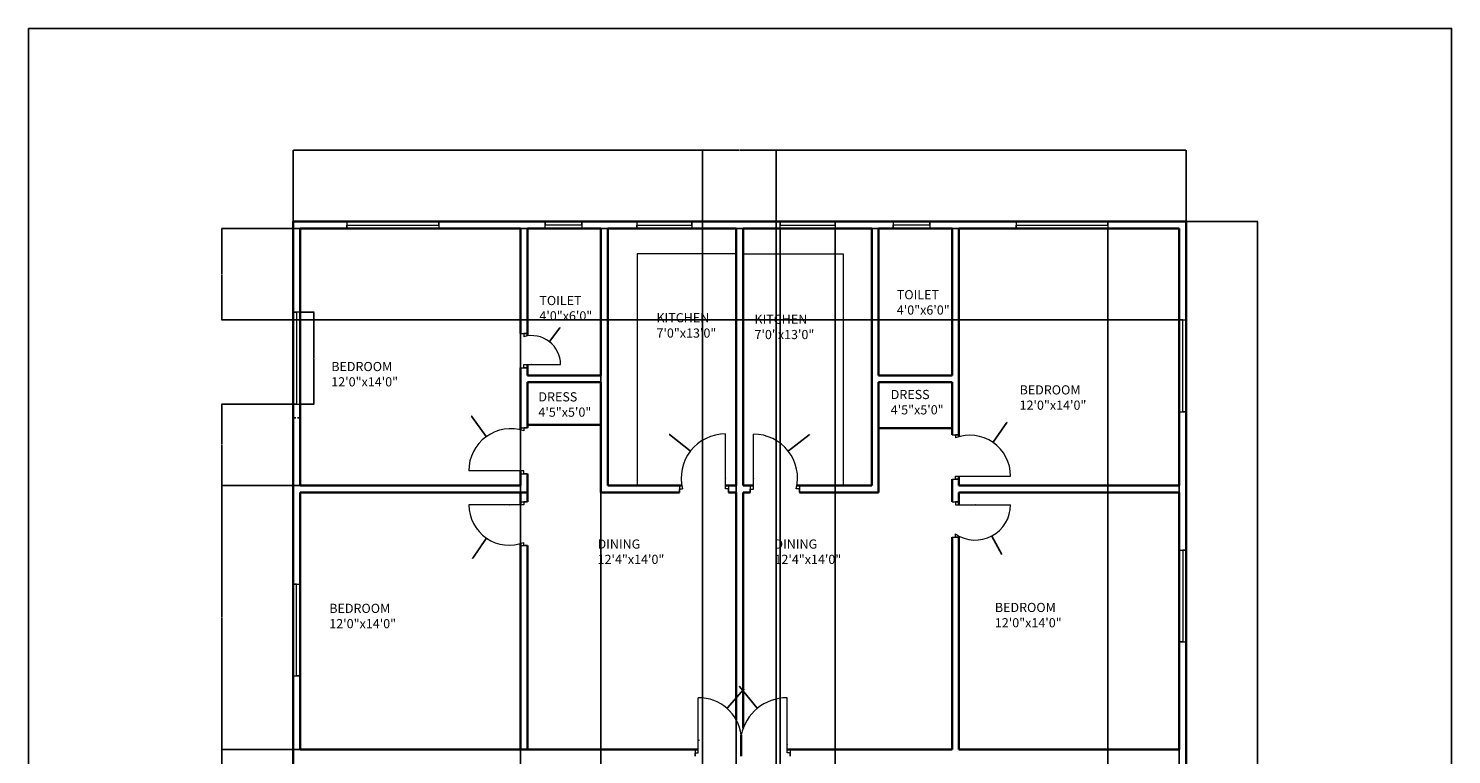
# Model space of a CAD drawing. Units: inches. Extents: x 1865 to 2795, y 1308 to 2437.
# Tile 3 of 3: x 1865 to 2795, y 1962 to 2437. Entities that reach past the tile are written whole.
import ezdxf

# ---------------------------------------------------------------- set-up
doc = ezdxf.new("R2010")
doc.units = ezdxf.units.IN
for name, color, linetype, lineweight in [('A-ANNO-DIMS', 2, 'Continuous', 18), ('A-ANNO-TTLB', 7, 'Continuous', 25), ('A-AREA-IDEN', 7, 'Continuous', 18), ('A-DOOR', 3, 'Continuous', 18), ('A-FLOR-CASE', 8, 'Continuous', 18), ('A-GLAZ', 4, 'Continuous', 18), ('A-WALL', 7, 'Continuous', 35)]:
    doc.layers.add(name, color=color, linetype=linetype, lineweight=lineweight)
doc.styles.get("Standard").update_dxf_attribs({"font": 'arial.ttf'})
doc.dimstyles.get("Standard").update_dxf_attribs({"dimtxt": 0.18, "dimasz": 0.18, "dimexe": 0.18, "dimexo": 0.0625, "dimgap": 0.09, "dimtad": 0, "dimtih": 1, "dimtoh": 1, "dimdec": 4, "dimzin": 0, "dimdsep": 46, "dimtxsty": 'Standard', "dimcen": 0.09, "dimadec": 0, "dimazin": 0, "dimtfac": 1, "dimtdec": 4, "dimtofl": 0, "dimtmove": 0, "dimatfit": 3, "dimfxl": 1, "dimtolj": 1, "dimtzin": 0, "dimarcsym": 0})

# ---------------------------------------------------------------- blocks, each defined once
blk = doc.blocks.new('WIN-60IN')
for p, q in [((0, 4.5), (0, 0)), ((0, 0), (0, 2.25)), ((0, 2.25), (60, 2.25)), ((60, 2.25), (60, 4.5)), ((60, 4.5), (60, 0))]:
    blk.add_line(p, q)
blk = doc.blocks.new('WIN-60IN-ALT')
for p, q in [((4.5, 60), (0, 60)), ((0, 60), (2.25, 60)), ((2.25, 60), (2.25, 0)), ((2.25, 0), (0, 0)), ((0, 0), (4.5, 0))]:
    blk.add_line(p, q)
blk = doc.blocks.new('*D8')
at = {"layer": 'A-ANNO-DIMS', "color": 0, "lineweight": -2, "transparency": 16777216}
for p, q in [((2042.9, 2251.4), (2052.02, 2251.4)), ((2051.84, 2251.22), (2051.84, 2221.58)), ((2051.84, 2191.58), (2051.84, 2221.21)), ((2042.9, 2191.4), (2052.02, 2191.4))]:
    blk.add_line(p, q, dxfattribs=at)
at = {"layer": 'A-ANNO-DIMS', "color": 0, "transparency": 16777216}
for points in [[(2051.81, 2251.22), (2051.87, 2251.22), (2051.84, 2251.4)], [(2051.81, 2191.58), (2051.87, 2191.58), (2051.84, 2191.4)]]:
    blk.add_solid(points, dxfattribs=at)
at = {"layer": 'Defpoints', "color": 0, "transparency": 16777216}
for p in [(2042.84, 2251.4), (2051.84, 2251.4), (2042.84, 2191.4)]:
    blk.add_point(p, dxfattribs=at)
at = {"layer": 'A-ANNO-DIMS', "color": 0, "transparency": 16777216, "insert": (2051.84, 2221.4), "char_height": 0.18, "attachment_point": 5}
blk.add_mtext('\\A1;ALT. WINDOW 60 TYP.', dxfattribs=at)
blk = doc.blocks.new('*D9')
at = {"layer": 'A-ANNO-DIMS', "color": 0, "lineweight": -2, "transparency": 16777216}
for p, q in [((2038.34, 2191.34), (2038.34, 2182.22)), ((2042.84, 2191.34), (2042.84, 2182.22)), ((2038.52, 2182.4), (2040.13, 2182.4)), ((2042.66, 2182.4), (2041.05, 2182.4))]:
    blk.add_line(p, q, dxfattribs=at)
at = {"layer": 'A-ANNO-DIMS', "color": 0, "transparency": 16777216}
for points in [[(2038.52, 2182.43), (2038.52, 2182.37), (2038.34, 2182.4)], [(2042.66, 2182.43), (2042.66, 2182.37), (2042.84, 2182.4)]]:
    blk.add_solid(points, dxfattribs=at)
at = {"layer": 'Defpoints', "color": 0, "transparency": 16777216}
for p in [(2038.34, 2191.4), (2042.84, 2191.4), (2042.84, 2182.4)]:
    blk.add_point(p, dxfattribs=at)
at = {"layer": 'A-ANNO-DIMS', "color": 0, "transparency": 16777216, "insert": (2040.59, 2182.4), "char_height": 0.18, "attachment_point": 5}
blk.add_mtext('\\A1;5 TYP.', dxfattribs=at)
blk = doc.blocks.new('*D10')
at = {"layer": 'A-ANNO-DIMS', "color": 0, "lineweight": -2, "transparency": 16777216}
for p, q in [((2038.34, 2310.72), (2038.34, 2357.44)), ((2038.52, 2357.26), (2329.69, 2357.26)), ((2621.66, 2357.26), (2330.48, 2357.26)), ((2621.84, 2310.72), (2621.84, 2357.44))]:
    blk.add_line(p, q, dxfattribs=at)
at = {"layer": 'A-ANNO-DIMS', "color": 0, "transparency": 16777216}
for points in [[(2038.52, 2357.29), (2038.52, 2357.23), (2038.34, 2357.26)], [(2621.66, 2357.29), (2621.66, 2357.23), (2621.84, 2357.26)]]:
    blk.add_solid(points, dxfattribs=at)
at = {"layer": 'Defpoints', "color": 0, "transparency": 16777216}
for p in [(2621.84, 2357.26), (2038.34, 2310.66), (2621.84, 2310.66)]:
    blk.add_point(p, dxfattribs=at)
at = {"layer": 'A-ANNO-DIMS', "color": 0, "transparency": 16777216, "insert": (2330.09, 2357.26), "char_height": 0.18, "attachment_point": 5}
blk.add_mtext('\\A1;583.5', dxfattribs=at)
blk = doc.blocks.new('*D11')
at = {"layer": 'A-ANNO-DIMS', "color": 0, "lineweight": -2, "transparency": 16777216}
for p, q in [((2621.9, 2310.66), (2668.62, 2310.66)), ((2668.44, 2310.48), (2668.44, 1911.09)), ((2668.44, 1511.34), (2668.44, 1910.72)), ((2621.9, 1511.16), (2668.62, 1511.16))]:
    blk.add_line(p, q, dxfattribs=at)
at = {"layer": 'A-ANNO-DIMS', "color": 0, "transparency": 16777216}
for points in [[(2668.41, 2310.48), (2668.47, 2310.48), (2668.44, 2310.66)], [(2668.41, 1511.34), (2668.47, 1511.34), (2668.44, 1511.16)]]:
    blk.add_solid(points, dxfattribs=at)
at = {"layer": 'Defpoints', "color": 0, "transparency": 16777216}
for p in [(2621.84, 2310.66), (2668.44, 2310.66), (2621.84, 1511.16)]:
    blk.add_point(p, dxfattribs=at)
at = {"layer": 'A-ANNO-DIMS', "color": 0, "transparency": 16777216, "insert": (2668.44, 1910.91), "char_height": 0.18, "attachment_point": 5}
blk.add_mtext('\\A1;799.5', dxfattribs=at)
blk = doc.blocks.new('*D12')
at = {"layer": 'A-ANNO-DIMS', "color": 0, "lineweight": -2, "transparency": 16777216}
for p, q in [((2038.34, 2310.59), (2038.34, 1341.86)), ((2186.84, 2306.09), (2186.84, 1341.86)), ((2038.52, 1342.04), (2112.2, 1342.04)), ((2186.66, 1342.04), (2112.97, 1342.04))]:
    blk.add_line(p, q, dxfattribs=at)
at = {"layer": 'A-ANNO-DIMS', "color": 0, "transparency": 16777216}
for points in [[(2038.52, 1342.07), (2038.52, 1342.01), (2038.34, 1342.04)], [(2186.66, 1342.07), (2186.66, 1342.01), (2186.84, 1342.04)]]:
    blk.add_solid(points, dxfattribs=at)
at = {"layer": 'Defpoints', "color": 0, "transparency": 16777216}
for p in [(2038.34, 2310.66), (2186.84, 2306.16), (2186.84, 1342.04)]:
    blk.add_point(p, dxfattribs=at)
at = {"layer": 'A-ANNO-DIMS', "color": 0, "transparency": 16777216, "insert": (2112.59, 1342.04), "char_height": 0.18, "attachment_point": 5}
blk.add_mtext('\\A1;148.5', dxfattribs=at)
blk = doc.blocks.new('*D13')
at = {"layer": 'A-ANNO-DIMS', "color": 0, "lineweight": -2, "transparency": 16777216}
for p, q in [((2186.84, 2306.09), (2186.84, 1341.86)), ((2239.34, 2306.09), (2239.34, 1341.86)), ((2187.02, 1342.04), (2212.76, 1342.04)), ((2239.16, 1342.04), (2213.41, 1342.04))]:
    blk.add_line(p, q, dxfattribs=at)
at = {"layer": 'A-ANNO-DIMS', "color": 0, "transparency": 16777216}
for points in [[(2187.02, 1342.07), (2187.02, 1342.01), (2186.84, 1342.04)], [(2239.16, 1342.07), (2239.16, 1342.01), (2239.34, 1342.04)]]:
    blk.add_solid(points, dxfattribs=at)
at = {"layer": 'Defpoints', "color": 0, "transparency": 16777216}
for p in [(2186.84, 2306.16), (2239.34, 2306.16), (2239.34, 1342.04)]:
    blk.add_point(p, dxfattribs=at)
at = {"layer": 'A-ANNO-DIMS', "color": 0, "transparency": 16777216, "insert": (2213.09, 1342.04), "char_height": 0.18, "attachment_point": 5}
blk.add_mtext('\\A1;52.5', dxfattribs=at)
blk = doc.blocks.new('*D14')
at = {"layer": 'A-ANNO-DIMS', "color": 0, "lineweight": -2, "transparency": 16777216}
for p, q in [((2239.34, 2306.09), (2239.34, 1341.86)), ((2327.84, 2306.09), (2327.84, 1341.86)), ((2239.52, 1342.04), (2283.26, 1342.04)), ((2327.66, 1342.04), (2283.91, 1342.04))]:
    blk.add_line(p, q, dxfattribs=at)
at = {"layer": 'A-ANNO-DIMS', "color": 0, "transparency": 16777216}
for points in [[(2239.52, 1342.07), (2239.52, 1342.01), (2239.34, 1342.04)], [(2327.66, 1342.07), (2327.66, 1342.01), (2327.84, 1342.04)]]:
    blk.add_solid(points, dxfattribs=at)
at = {"layer": 'Defpoints', "color": 0, "transparency": 16777216}
for p in [(2239.34, 2306.16), (2327.84, 2306.16), (2327.84, 1342.04)]:
    blk.add_point(p, dxfattribs=at)
at = {"layer": 'A-ANNO-DIMS', "color": 0, "transparency": 16777216, "insert": (2283.59, 1342.04), "char_height": 0.18, "attachment_point": 5}
blk.add_mtext('\\A1;88.5', dxfattribs=at)
blk = doc.blocks.new('*D15')
at = {"layer": 'A-ANNO-DIMS', "color": 0, "lineweight": -2, "transparency": 16777216}
for p, q in [((2570.72, 2306.09), (2570.72, 1341.86)), ((2617.34, 2306.09), (2617.34, 1341.86)), ((2570.9, 1342.04), (2593.65, 1342.04)), ((2617.16, 1342.04), (2594.41, 1342.04))]:
    blk.add_line(p, q, dxfattribs=at)
at = {"layer": 'A-ANNO-DIMS', "color": 0, "transparency": 16777216}
for points in [[(2570.9, 1342.07), (2570.9, 1342.01), (2570.72, 1342.04)], [(2617.16, 1342.07), (2617.16, 1342.01), (2617.34, 1342.04)]]:
    blk.add_solid(points, dxfattribs=at)
at = {"layer": 'Defpoints', "color": 0, "transparency": 16777216}
for p in [(2570.72, 2306.16), (2617.34, 2306.16), (2617.34, 1342.04)]:
    blk.add_point(p, dxfattribs=at)
at = {"layer": 'A-ANNO-DIMS', "color": 0, "transparency": 16777216, "insert": (2594.03, 1342.04), "char_height": 0.18, "attachment_point": 5}
blk.add_mtext('\\A1;46.61', dxfattribs=at)
blk = doc.blocks.new('*D16')
at = {"layer": 'A-ANNO-DIMS', "color": 0, "lineweight": -2, "transparency": 16777216}
for p, q in [((2617.28, 2306.16), (1991.56, 2306.16)), ((1991.74, 2305.98), (1991.74, 2276.44)), ((1991.74, 2246.54), (1991.74, 2276.08)), ((2617.28, 2246.36), (1991.56, 2246.36))]:
    blk.add_line(p, q, dxfattribs=at)
at = {"layer": 'A-ANNO-DIMS', "color": 0, "transparency": 16777216}
for points in [[(1991.71, 2305.98), (1991.77, 2305.98), (1991.74, 2306.16)], [(1991.71, 2246.54), (1991.77, 2246.54), (1991.74, 2246.36)]]:
    blk.add_solid(points, dxfattribs=at)
at = {"layer": 'Defpoints', "color": 0, "transparency": 16777216}
for p in [(1991.74, 2306.16), (2617.34, 2306.16), (2617.34, 2246.36)]:
    blk.add_point(p, dxfattribs=at)
at = {"layer": 'A-ANNO-DIMS', "color": 0, "transparency": 16777216, "insert": (1991.74, 2276.26), "char_height": 0.18, "attachment_point": 5}
blk.add_mtext('\\A1;59.79', dxfattribs=at)
blk = doc.blocks.new('*D17')
at = {"layer": 'A-ANNO-DIMS', "color": 0, "lineweight": -2, "transparency": 16777216}
for p, q in [((2038.28, 2191.4), (1991.56, 2191.4)), ((1991.74, 2191.22), (1991.74, 2164.96)), ((1991.74, 2138.34), (1991.74, 2164.6)), ((2042.78, 2138.16), (1991.56, 2138.16))]:
    blk.add_line(p, q, dxfattribs=at)
at = {"layer": 'A-ANNO-DIMS', "color": 0, "transparency": 16777216}
for points in [[(1991.71, 2191.22), (1991.77, 2191.22), (1991.74, 2191.4)], [(1991.71, 2138.34), (1991.77, 2138.34), (1991.74, 2138.16)]]:
    blk.add_solid(points, dxfattribs=at)
at = {"layer": 'Defpoints', "color": 0, "transparency": 16777216}
for p in [(1991.74, 2191.4), (2038.34, 2191.4), (2042.84, 2138.16)]:
    blk.add_point(p, dxfattribs=at)
at = {"layer": 'A-ANNO-DIMS', "color": 0, "transparency": 16777216, "insert": (1991.74, 2164.78), "char_height": 0.18, "attachment_point": 5}
blk.add_mtext('\\A1;53.24', dxfattribs=at)
blk = doc.blocks.new('*D18')
at = {"layer": 'A-ANNO-DIMS', "color": 0, "lineweight": -2, "transparency": 16777216}
for p, q in [((2356.56, 2306.09), (2356.56, 1341.86)), ((2392.56, 2306.09), (2392.56, 1341.86)), ((2356.74, 1342.04), (2374.34, 1342.04)), ((2392.38, 1342.04), (2374.78, 1342.04))]:
    blk.add_line(p, q, dxfattribs=at)
at = {"layer": 'A-ANNO-DIMS', "color": 0, "transparency": 16777216}
for points in [[(2356.74, 1342.07), (2356.74, 1342.01), (2356.56, 1342.04)], [(2392.38, 1342.07), (2392.38, 1342.01), (2392.56, 1342.04)]]:
    blk.add_solid(points, dxfattribs=at)
at = {"layer": 'Defpoints', "color": 0, "transparency": 16777216}
for p in [(2356.56, 2306.16), (2392.56, 2306.16), (2392.56, 1342.04)]:
    blk.add_point(p, dxfattribs=at)
at = {"layer": 'A-ANNO-DIMS', "color": 0, "transparency": 16777216, "insert": (2374.56, 1342.04), "char_height": 0.18, "attachment_point": 5}
blk.add_mtext('\\A1;36', dxfattribs=at)
blk = doc.blocks.new('*D19')
at = {"layer": 'A-ANNO-DIMS', "color": 0, "lineweight": -2, "transparency": 16777216}
for p, q in [((2305.85, 1520.22), (2305.85, 2357.44)), ((2306.03, 2357.26), (2329.63, 2357.26)), ((2353.67, 2357.26), (2330.08, 2357.26)), ((2353.85, 1520.22), (2353.85, 2357.44))]:
    blk.add_line(p, q, dxfattribs=at)
at = {"layer": 'A-ANNO-DIMS', "color": 0, "transparency": 16777216}
for points in [[(2306.03, 2357.29), (2306.03, 2357.23), (2305.85, 2357.26)], [(2353.67, 2357.29), (2353.67, 2357.23), (2353.85, 2357.26)]]:
    blk.add_solid(points, dxfattribs=at)
at = {"layer": 'Defpoints', "color": 0, "transparency": 16777216}
for p in [(2353.85, 2357.26), (2305.85, 1520.16), (2353.85, 1520.16)]:
    blk.add_point(p, dxfattribs=at)
at = {"layer": 'A-ANNO-DIMS', "color": 0, "transparency": 16777216, "insert": (2329.85, 2357.26), "char_height": 0.18, "attachment_point": 5}
blk.add_mtext('\\A1;48', dxfattribs=at)
blk = doc.blocks.new('*D23')
at = {"layer": 'A-ANNO-DIMS', "color": 0, "lineweight": -2, "transparency": 16777216}
for p, q in [((2042.78, 1965.66), (1991.56, 1965.66)), ((1991.74, 1965.48), (1991.74, 1939.59)), ((1991.74, 1913.34), (1991.74, 1939.22)), ((2042.78, 1913.16), (1991.56, 1913.16))]:
    blk.add_line(p, q, dxfattribs=at)
at = {"layer": 'A-ANNO-DIMS', "color": 0, "transparency": 16777216}
for points in [[(1991.71, 1965.48), (1991.77, 1965.48), (1991.74, 1965.66)], [(1991.71, 1913.34), (1991.77, 1913.34), (1991.74, 1913.16)]]:
    blk.add_solid(points, dxfattribs=at)
at = {"layer": 'Defpoints', "color": 0, "transparency": 16777216}
for p in [(1991.74, 1965.66), (2042.84, 1965.66), (2042.84, 1913.16)]:
    blk.add_point(p, dxfattribs=at)
at = {"layer": 'A-ANNO-DIMS', "color": 0, "transparency": 16777216, "insert": (1991.74, 1939.41), "char_height": 0.18, "attachment_point": 5}
blk.add_mtext('\\A1;52.5', dxfattribs=at)
blk = doc.blocks.new('*D24')
at = {"layer": 'A-ANNO-DIMS', "color": 0, "lineweight": -2, "transparency": 16777216}
for p, q in [((2042.78, 2138.16), (1991.56, 2138.16)), ((1991.74, 2137.98), (1991.74, 2052.09)), ((1991.74, 1965.84), (1991.74, 2051.72)), ((2042.78, 1965.66), (1991.56, 1965.66))]:
    blk.add_line(p, q, dxfattribs=at)
at = {"layer": 'A-ANNO-DIMS', "color": 0, "transparency": 16777216}
for points in [[(1991.71, 2137.98), (1991.77, 2137.98), (1991.74, 2138.16)], [(1991.71, 1965.84), (1991.77, 1965.84), (1991.74, 1965.66)]]:
    blk.add_solid(points, dxfattribs=at)
at = {"layer": 'Defpoints', "color": 0, "transparency": 16777216}
for p in [(1991.74, 2138.16), (2042.84, 2138.16), (2042.84, 1965.66)]:
    blk.add_point(p, dxfattribs=at)
at = {"layer": 'A-ANNO-DIMS', "color": 0, "transparency": 16777216, "insert": (1991.74, 2051.91), "char_height": 0.18, "attachment_point": 5}
blk.add_mtext('\\A1;172.5', dxfattribs=at)
blk = doc.blocks.new('*D29')
at = {"layer": 'A-ANNO-DIMS', "color": 0, "lineweight": -2, "transparency": 16777216}
for p, q in [((2329.85, 2006.74), (2330.03, 2006.74)), ((2330.03, 2006.74), (2341.54, 1992.65)), ((2360.93, 1968.78), (2361.11, 1968.78)), ((2361.02, 1968.69), (2361.02, 1968.87))]:
    blk.add_line(p, q, dxfattribs=at)
at = {"layer": 'A-ANNO-DIMS', "color": 0, "transparency": 16777216}
blk.add_solid([(2341.56, 1992.66), (2341.51, 1992.63), (2341.65, 1992.51)], dxfattribs=at)
at = {"layer": 'Defpoints', "color": 0, "transparency": 16777216}
for p in [(2341.65, 1992.51), (2361.02, 1968.78)]:
    blk.add_point(p, dxfattribs=at)
at = {"layer": 'A-ANNO-DIMS', "color": 0, "transparency": 16777216, "insert": (2329.37, 2006.74), "char_height": 0.18, "attachment_point": 5}
blk.add_mtext('\\A1;R30.63', dxfattribs=at)
blk = doc.blocks.new('*D32')
at = {"layer": 'A-ANNO-DIMS', "color": 0, "lineweight": -2, "transparency": 16777216}
for p, q in [((2375.42, 2171.32), (2361.91, 2160.75)), ((2375.6, 2171.32), (2375.42, 2171.32)), ((2338.94, 2142.84), (2339.12, 2142.84)), ((2339.03, 2142.75), (2339.03, 2142.93))]:
    blk.add_line(p, q, dxfattribs=at)
at = {"layer": 'A-ANNO-DIMS', "color": 0, "transparency": 16777216}
blk.add_solid([(2361.9, 2160.78), (2361.93, 2160.73), (2361.77, 2160.64)], dxfattribs=at)
at = {"layer": 'Defpoints', "color": 0, "transparency": 16777216}
for p in [(2361.77, 2160.64), (2339.03, 2142.84)]:
    blk.add_point(p, dxfattribs=at)
at = {"layer": 'A-ANNO-DIMS', "color": 0, "transparency": 16777216, "insert": (2376.08, 2171.32), "char_height": 0.18, "attachment_point": 5}
blk.add_mtext('\\A1;R28.88', dxfattribs=at)
blk = doc.blocks.new('*D33')
at = {"layer": 'A-ANNO-DIMS', "color": 0, "lineweight": -2, "transparency": 16777216}
for p, q in [((2284.11, 2171.38), (2284.29, 2171.38)), ((2284.29, 2171.38), (2297.83, 2160.86)), ((2320.68, 2143.03), (2320.86, 2143.03)), ((2320.77, 2142.94), (2320.77, 2143.12))]:
    blk.add_line(p, q, dxfattribs=at)
at = {"layer": 'A-ANNO-DIMS', "color": 0, "transparency": 16777216}
blk.add_solid([(2297.85, 2160.89), (2297.81, 2160.84), (2297.97, 2160.75)], dxfattribs=at)
at = {"layer": 'Defpoints', "color": 0, "transparency": 16777216}
for p in [(2297.97, 2160.75), (2320.77, 2143.03)]:
    blk.add_point(p, dxfattribs=at)
at = {"layer": 'A-ANNO-DIMS', "color": 0, "transparency": 16777216, "insert": (2283.56, 2171.38), "char_height": 0.18, "attachment_point": 5}
blk.add_mtext('\\A1;R28.874', dxfattribs=at)
blk = doc.blocks.new('*D37')
at = {"layer": 'A-ANNO-DIMS', "color": 0, "lineweight": -2, "transparency": 16777216}
for p, q in [((2332.69, 2005.08), (2321.84, 1992.68)), ((2332.87, 2005.08), (2332.69, 2005.08)), ((2303.35, 1971.65), (2303.53, 1971.65)), ((2303.44, 1971.56), (2303.44, 1971.74))]:
    blk.add_line(p, q, dxfattribs=at)
at = {"layer": 'A-ANNO-DIMS', "color": 0, "transparency": 16777216}
blk.add_solid([(2321.82, 1992.7), (2321.86, 1992.66), (2321.72, 1992.54)], dxfattribs=at)
at = {"layer": 'Defpoints', "color": 0, "transparency": 16777216}
for p in [(2321.72, 1992.54), (2303.44, 1971.65)]:
    blk.add_point(p, dxfattribs=at)
at = {"layer": 'A-ANNO-DIMS', "color": 0, "transparency": 16777216, "insert": (2333.54, 2005.08), "char_height": 0.18, "attachment_point": 5}
blk.add_mtext('\\A1;2X R27.76', dxfattribs=at)
blk = doc.blocks.new('*D39')
at = {"layer": 'A-ANNO-DIMS', "color": 0, "lineweight": -2, "transparency": 16777216}
for p, q in [((2154.58, 2183.38), (2154.76, 2183.38)), ((2154.76, 2183.38), (2164.32, 2170.19)), ((2180.46, 2147.81), (2180.64, 2147.81)), ((2180.55, 2147.72), (2180.55, 2147.9))]:
    blk.add_line(p, q, dxfattribs=at)
at = {"layer": 'A-ANNO-DIMS', "color": 0, "transparency": 16777216}
blk.add_solid([(2164.35, 2170.2), (2164.3, 2170.17), (2164.43, 2170.04)], dxfattribs=at)
at = {"layer": 'Defpoints', "color": 0, "transparency": 16777216}
for p in [(2164.43, 2170.04), (2180.55, 2147.81)]:
    blk.add_point(p, dxfattribs=at)
at = {"layer": 'A-ANNO-DIMS', "color": 0, "transparency": 16777216, "insert": (2154.03, 2183.38), "char_height": 0.18, "attachment_point": 5}
blk.add_mtext('\\A1;R27.464', dxfattribs=at)
blk = doc.blocks.new('*D40')
at = {"layer": 'A-ANNO-DIMS', "color": 0, "lineweight": -2, "transparency": 16777216}
for p, q in [((2504.69, 2179.37), (2495.72, 2166.39)), ((2504.87, 2179.37), (2504.69, 2179.37)), ((2480.4, 2144.36), (2480.58, 2144.36)), ((2480.49, 2144.27), (2480.49, 2144.45))]:
    blk.add_line(p, q, dxfattribs=at)
at = {"layer": 'A-ANNO-DIMS', "color": 0, "transparency": 16777216}
blk.add_solid([(2495.69, 2166.4), (2495.74, 2166.37), (2495.61, 2166.24)], dxfattribs=at)
at = {"layer": 'Defpoints', "color": 0, "transparency": 16777216}
for p in [(2495.61, 2166.24), (2480.49, 2144.36)]:
    blk.add_point(p, dxfattribs=at)
at = {"layer": 'A-ANNO-DIMS', "color": 0, "transparency": 16777216, "insert": (2505.28, 2179.37), "char_height": 0.18, "attachment_point": 5}
blk.add_mtext('\\A1;R26.6', dxfattribs=at)
blk = doc.blocks.new('*D41')
at = {"layer": 'A-ANNO-DIMS', "color": 0, "lineweight": -2, "transparency": 16777216}
for p, q in [((2179.43, 2125.54), (2179.61, 2125.54)), ((2179.52, 2125.45), (2179.52, 2125.63)), ((2155.63, 2090.64), (2164.49, 2103.58)), ((2155.45, 2090.64), (2155.63, 2090.64))]:
    blk.add_line(p, q, dxfattribs=at)
at = {"layer": 'A-ANNO-DIMS', "color": 0, "transparency": 16777216}
blk.add_solid([(2164.46, 2103.6), (2164.51, 2103.56), (2164.59, 2103.73)], dxfattribs=at)
at = {"layer": 'Defpoints', "color": 0, "transparency": 16777216}
for p in [(2179.52, 2125.54), (2164.59, 2103.73)]:
    blk.add_point(p, dxfattribs=at)
at = {"layer": 'A-ANNO-DIMS', "color": 0, "transparency": 16777216, "insert": (2154.97, 2090.64), "char_height": 0.18, "attachment_point": 5}
blk.add_mtext('\\A1;R26.43', dxfattribs=at)
blk = doc.blocks.new('*D42')
at = {"layer": 'A-ANNO-DIMS', "color": 0, "lineweight": -2, "transparency": 16777216}
for p, q in [((2483.95, 2125.54), (2484.13, 2125.54)), ((2484.04, 2125.45), (2484.04, 2125.63)), ((2501.3, 2092.95), (2494.91, 2105.01)), ((2501.48, 2092.95), (2501.3, 2092.95))]:
    blk.add_line(p, q, dxfattribs=at)
at = {"layer": 'A-ANNO-DIMS', "color": 0, "transparency": 16777216}
blk.add_solid([(2494.94, 2105.02), (2494.88, 2104.99), (2494.83, 2105.17)], dxfattribs=at)
at = {"layer": 'Defpoints', "color": 0, "transparency": 16777216}
for p in [(2484.04, 2125.54), (2494.83, 2105.17)]:
    blk.add_point(p, dxfattribs=at)
at = {"layer": 'A-ANNO-DIMS', "color": 0, "transparency": 16777216, "insert": (2501.96, 2092.95), "char_height": 0.18, "attachment_point": 5}
blk.add_mtext('\\A1;R23.05', dxfattribs=at)
blk = doc.blocks.new('*D47')
at = {"layer": 'A-ANNO-DIMS', "color": 0, "lineweight": -2, "transparency": 16777216}
for p, q in [((2212.52, 2241.29), (2205.73, 2232.38)), ((2212.7, 2241.29), (2212.52, 2241.29)), ((2194.03, 2217.15), (2194.21, 2217.15)), ((2194.12, 2217.06), (2194.12, 2217.24))]:
    blk.add_line(p, q, dxfattribs=at)
at = {"layer": 'A-ANNO-DIMS', "color": 0, "transparency": 16777216}
blk.add_solid([(2205.7, 2232.4), (2205.75, 2232.36), (2205.62, 2232.24)], dxfattribs=at)
at = {"layer": 'Defpoints', "color": 0, "transparency": 16777216}
for p in [(2205.62, 2232.24), (2194.12, 2217.15)]:
    blk.add_point(p, dxfattribs=at)
at = {"layer": 'A-ANNO-DIMS', "color": 0, "transparency": 16777216, "insert": (2213.18, 2241.29), "char_height": 0.18, "attachment_point": 5}
blk.add_mtext('\\A1;R18.97', dxfattribs=at)

msp = doc.modelspace()

# ---------------------------------------------------------------- linework, layer by layer
at = {"layer": 'A-ANNO-TTLB'}
msp.add_lwpolyline([(1865.3404, 2436.9121), (2795.2369, 2436.9121), (2795.2369, 1308.3367), (1865.3404, 1308.3367)], close=True, dxfattribs=at)
at = {"layer": 'A-DOOR'}
for p, q in [((2186.8379, 2237.4394), (2191.3379, 2237.4394)), ((2191.3379, 2237.4394), (2189.0879, 2237.4394)), ((2189.0879, 2237.4394), (2189.0879, 2235.4394)), ((2186.8379, 2215.1471), (2191.3379, 2215.1471)), ((2189.0879, 2215.1471), (2189.0879, 2217.1471)), ((2189.0879, 2217.1471), (2213.0879, 2217.1471)), ((2191.3379, 2215.1471), (2189.0879, 2215.1471)), ((2186.8379, 2175.9108), (2191.3379, 2175.9108)), ((2191.3379, 2175.9108), (2189.0879, 2175.9108)), ((2189.0879, 2175.9108), (2189.0879, 2173.9108)), ((2320.7668, 2135.9064), (2320.7668, 2171.9064)), ((2339.0309, 2135.7192), (2339.0309, 2171.7192)), ((2468.8379, 2171.2409), (2473.3379, 2171.2409)), ((2473.3379, 2171.2409), (2471.0879, 2171.2409)), ((2471.0879, 2171.2409), (2471.0879, 2169.2409)), ((2189.0879, 2147.8064), (2153.0879, 2147.8064)), ((2186.8379, 2145.8064), (2191.3379, 2145.8064)), ((2189.0879, 2145.8064), (2189.0879, 2147.8064)), ((2191.3379, 2145.8064), (2189.0879, 2145.8064)), ((2468.8379, 2142.3558), (2473.3379, 2142.3558)), ((2471.0879, 2142.3558), (2471.0879, 2144.3558)), ((2471.0879, 2144.3558), (2507.0879, 2144.3558)), ((2473.3379, 2142.3558), (2471.0879, 2142.3558)), ((2290.7858, 2138.1564), (2290.7858, 2133.6564)), ((2290.7858, 2133.6564), (2290.7858, 2135.9064)), ((2290.7858, 2135.9064), (2292.7858, 2135.9064)), ((2322.7668, 2135.9064), (2320.7668, 2135.9064)), ((2322.7668, 2138.1564), (2322.7668, 2133.6564)), ((2322.7668, 2133.6564), (2322.7668, 2135.9064)), ((2337.0309, 2138.1564), (2337.0309, 2135.0328)), ((2337.0309, 2133.6564), (2337.0309, 2135.7192)), ((2337.0309, 2135.7192), (2339.0309, 2135.7192)), ((2337.0309, 2135.0328), (2337.0309, 2133.6564)), ((2369.07, 2135.9064), (2367.07, 2135.9064)), ((2369.07, 2138.1564), (2369.07, 2133.6564)), ((2369.07, 2133.6564), (2369.07, 2135.9064)), ((2189.0879, 2125.5426), (2153.0879, 2125.5426)), ((2186.8379, 2127.5426), (2191.3379, 2127.5426)), ((2191.3379, 2127.5426), (2189.0879, 2127.5426)), ((2189.0879, 2127.5426), (2189.0879, 2125.5426)), ((2468.8379, 2127.5371), (2473.3379, 2127.5371)), ((2473.3379, 2127.5371), (2471.0879, 2127.5371)), ((2471.0879, 2127.5371), (2471.0879, 2127.5371)), ((2471.0879, 2127.5371), (2471.0879, 2125.5371)), ((2471.0879, 2125.5371), (2507.0879, 2125.5371)), ((2468.8379, 2104.4669), (2473.3379, 2104.4669)), ((2471.0879, 2104.4669), (2471.0879, 2106.4669)), ((2473.3379, 2104.4669), (2471.0879, 2104.4669)), ((2186.8379, 2098.9035), (2191.3379, 2098.9035)), ((2189.0879, 2098.9035), (2189.0879, 2100.9035)), ((2191.3379, 2098.9035), (2189.0879, 2098.9035)), ((2303.0168, 1963.4064), (2303.0168, 1999.4064)), ((2361.0176, 1963.4064), (2361.0176, 1999.4064)), ((2301.0168, 1965.6564), (2301.0168, 1961.1564)), ((2301.0168, 1961.1564), (2301.0168, 1963.4064)), ((2301.0168, 1963.4064), (2303.0168, 1963.4064)), ((2363.0176, 1963.4064), (2361.0176, 1963.4064)), ((2363.0176, 1965.6564), (2363.0176, 1961.1564)), ((2363.0176, 1961.1564), (2363.0176, 1963.4064))]:
    msp.add_line(p, q, dxfattribs=at)
for centre, radius, start, end in [((2194.1168, 2217.1471), 18.971, 360, 105.3721505), ((2180.5523, 2147.8064), 27.4645, 71.8934406, 180), ((2320.7668, 2143.0323), 28.8741, 90, 194.2877333), ((2339.0309, 2142.8364), 28.8828, 346.1173753, 90), ((2480.4869, 2144.3558), 26.601, 0, 110.6914414), ((2179.5196, 2125.5426), 26.4317, 180, 291.2230785), ((2484.0368, 2125.5371), 23.051, 235.8228252, 0), ((2303.4402, 1971.6481), 27.7616, 331.5011644, 331.5011645), ((2303.4402, 1971.6481), 27.7616, 6.7545, 90.8739372), ((2361.0176, 1968.777), 30.6295, 90, 168.4430965)]:
    msp.add_arc(centre, radius, start, end, dxfattribs=at)
at = {"layer": 'A-FLOR-CASE'}
for p, q in [((2327.8379, 2289.6138), (2263.2016, 2289.6138)), ((2263.2016, 2289.6138), (2263.2016, 2138.1564)), ((2332.3379, 2289.6138), (2397.596, 2289.6138)), ((2397.596, 2289.6138), (2397.596, 2138.1564))]:
    msp.add_line(p, q, dxfattribs=at)
at = {"layer": 'A-GLAZ'}
for p, q in [((2073.4318, 2310.6564), (2073.4318, 2306.1564)), ((2073.4318, 2306.1564), (2073.4318, 2308.4064)), ((2073.4318, 2308.4064), (2133.4318, 2308.4064)), ((2133.4318, 2308.4064), (2133.4318, 2310.6564)), ((2133.4318, 2310.6564), (2133.4318, 2306.8241)), ((2133.4318, 2306.8241), (2133.4318, 2306.1564)), ((2203.0284, 2309.5152), (2203.0284, 2310.6564)), ((2203.0284, 2310.6564), (2203.0284, 2308.1788)), ((2203.0284, 2306.1564), (2203.0284, 2309.5152)), ((2203.0284, 2308.1788), (2203.0284, 2308.5237)), ((2203.0284, 2308.5237), (2227.0284, 2308.5237)), ((2227.0284, 2308.5237), (2227.0284, 2310.6564)), ((2227.0284, 2310.6564), (2227.0284, 2306.1564)), ((2262.8123, 2310.6564), (2262.8123, 2306.1564)), ((2262.8123, 2306.1564), (2262.8123, 2308.4064)), ((2262.8123, 2308.4064), (2298.8123, 2308.4064)), ((2298.8123, 2308.4064), (2298.8123, 2310.6564)), ((2298.8123, 2310.6564), (2298.8123, 2306.1564)), ((2356.5618, 2306.1564), (2356.5618, 2310.6564)), ((2356.5618, 2310.6564), (2356.5618, 2308.4064)), ((2356.5618, 2308.4064), (2392.5618, 2308.4064)), ((2392.5618, 2308.4064), (2392.5618, 2310.6564)), ((2392.5618, 2310.6564), (2392.5618, 2306.1564)), ((2430.2913, 2310.6564), (2430.2913, 2307.881)), ((2430.2913, 2306.1564), (2430.2913, 2308.4996)), ((2430.2913, 2308.4996), (2454.2913, 2308.4996)), ((2430.2913, 2307.881), (2430.2913, 2306.1564)), ((2454.2913, 2308.4996), (2454.2913, 2310.6564)), ((2454.2913, 2310.6564), (2454.2913, 2306.1564))]:
    msp.add_line(p, q, dxfattribs=at)
at = {"layer": 'A-WALL'}
for p, q in [((2038.3379, 2310.6564), (2621.8379, 2310.6564)), ((2038.3379, 2310.6564), (2038.3379, 1511.1564)), ((2042.8379, 2306.1564), (2186.8379, 2306.1564)), ((2042.8379, 2306.1564), (2042.8379, 2138.1564)), ((2186.8379, 2306.1564), (2186.8379, 2237.4394)), ((2191.3379, 2306.1564), (2191.3379, 2235.9135)), ((2191.3379, 2306.1564), (2239.3379, 2306.1564)), ((2239.3379, 2306.1564), (2239.3379, 2210.1564)), ((2243.8379, 2306.1564), (2243.8379, 2138.1564)), ((2243.8379, 2306.1564), (2327.8379, 2306.1564)), ((2327.8379, 2306.1564), (2327.8379, 2138.1564)), ((2332.3379, 2306.1564), (2332.3379, 2138.1564)), ((2332.3379, 2306.1564), (2416.3379, 2306.1564)), ((2416.3379, 2306.1564), (2416.3379, 2138.1564)), ((2420.8379, 2306.1564), (2420.8379, 2210.1564)), ((2420.8379, 2306.1564), (2468.8379, 2306.1564)), ((2468.8379, 2306.1564), (2468.8379, 2210.1564)), ((2473.3379, 2306.1564), (2473.3379, 2169.9781)), ((2473.3379, 2306.1564), (2617.3379, 2306.1564)), ((2617.3379, 2306.1564), (2617.3379, 2138.1564)), ((2621.8379, 2310.6564), (2621.8379, 1511.1564)), ((2186.8379, 2215.1471), (2186.8379, 2174.5419)), ((2191.3379, 2217.1471), (2191.3379, 2210.1564)), ((2191.3379, 2210.1564), (2239.3379, 2210.1564)), ((2191.3379, 2205.6564), (2239.3379, 2205.6564)), ((2191.3379, 2205.6564), (2191.3379, 2175.9108)), ((2239.3379, 2205.6564), (2239.3379, 2133.6564)), ((2420.8379, 2210.1564), (2468.8379, 2210.1564)), ((2420.8379, 2205.6564), (2468.8379, 2205.6564)), ((2420.8379, 2205.6564), (2420.8379, 2133.6564)), ((2468.8379, 2205.6564), (2468.8379, 2171.2409)), ((2191.3379, 2177.7803), (2239.3379, 2177.7803)), ((2468.8379, 2175.5681), (2420.8379, 2175.5681)), ((2186.8379, 2147.8064), (2186.8379, 2138.1564)), ((2191.3379, 2145.8064), (2191.3379, 2127.5426)), ((2468.8379, 2142.3558), (2468.8379, 2127.5371)), ((2473.3379, 2144.3558), (2473.3379, 2138.1564)), ((2042.8379, 2138.1564), (2186.8379, 2138.1564)), ((2042.8379, 2133.6564), (2191.3379, 2133.6564)), ((2042.8379, 2133.6564), (2042.8379, 1965.6564)), ((2186.8379, 2133.6564), (2186.8379, 2125.5426)), ((2239.3379, 2133.6564), (2290.7858, 2133.6564)), ((2243.8379, 2138.1564), (2292.3073, 2138.1564)), ((2320.7668, 2138.1564), (2327.8379, 2138.1564)), ((2322.7668, 2133.6564), (2327.8379, 2133.6564)), ((2327.8379, 2133.6564), (2327.8379, 1984.8943)), ((2332.3379, 2138.1564), (2339.0309, 2138.1564)), ((2332.3379, 2133.6564), (2332.3379, 1979.5304)), ((2332.3379, 2133.6564), (2337.0309, 2133.6564)), ((2367.532, 2138.1564), (2416.3379, 2138.1564)), ((2369.07, 2133.6564), (2420.8379, 2133.6564)), ((2473.3379, 2138.1564), (2617.3379, 2138.1564)), ((2473.3379, 2133.6564), (2617.3379, 2133.6564)), ((2473.3379, 2133.6564), (2473.3379, 2125.5371)), ((2617.3379, 2133.6564), (2617.3379, 1965.6564)), ((2468.8379, 2104.4669), (2468.8379, 1965.6564)), ((2473.3379, 2105.1195), (2473.3379, 1965.6564)), ((2186.8379, 2100.1442), (2186.8379, 1965.6564)), ((2191.3379, 2098.9035), (2191.3379, 1965.6564)), ((2331.0091, 1974.9133), (2331.0091, 1961.1564)), ((2042.8379, 1965.6564), (2191.3379, 1965.6564)), ((2191.3379, 1965.6564), (2303.0168, 1965.6564)), ((2361.0176, 1965.6564), (2468.8379, 1965.6564)), ((2473.3379, 1965.6564), (2617.3379, 1965.6564))]:
    msp.add_line(p, q, dxfattribs=at)

# ---------------------------------------------------------------- block references
at = {"layer": 'A-GLAZ'}
for name, p in [('WIN-60IN', (2510.7249, 2306.156)), ('WIN-60IN-ALT', (2038.338, 2191.398))]:
    msp.add_blockref(name, p, dxfattribs=at)
at = {"layer": 'A-GLAZ', "rotation": 90}
for p in [(2621.8383, 2186.3643), (2042.8383, 2013.6728)]:
    msp.add_blockref('WIN-60IN', p, dxfattribs=at)
at = {"layer": 'A-GLAZ', "extrusion": (0, 0, -1), "zscale": -1, "rotation": 270}
msp.add_blockref('WIN-60IN', (-2621.8383, 2095.9865), dxfattribs=at)

# ---------------------------------------------------------------- texts
at = {"layer": 'A-AREA-IDEN', "char_height": 6, "attachment_point": 1}
for s, width, insert in [('TOILET\\P4\'0"x6\'0"', 102.663636, (2199.1928, 2262.0452)), ('TOILET\\P4\'0"x6\'0"', 91.44679, (2432.7557, 2265.8677)), ('KITCHEN\\P7\'0"x13\'0"', 129.893203, (2275.7071, 2250.8137)), ('KITCHEN\\P7\'0"x13\'0"', 104.560023, (2339.7571, 2249.8387)), ('BEDROOM\\P12\'0"x14\'0"', 244.26331, (2063.2119, 2218.9124)), ('DRESS\\P4\'5"x5\'0"', 141.45202, (2198.5641, 2199.111)), ('DRESS\\P4\'5"x5\'0"', 167.388868, (2428.7874, 2200.6379)), ('BEDROOM\\P12\'0"x14\'0"', 229.651123, (2512.9891, 2203.6556)), ('DINING\\P12\'4"x14\'0"', 115.598365, (2237.2186, 2102.8785)), ('DINING\\P12\'4"x14\'0"', 222.942588, (2352.817, 2102.8785)), ('BEDROOM\\P12\'0"x14\'0"', 256.4928, (2061.9091, 2060.8446)), ('BEDROOM\\P12\'0"x14\'0"', 222.251188, (2496.8265, 2061.4446))]:
    msp.add_mtext_dynamic_manual_height_columns(s, width=width, gutter_width=12.5, heights=[0], dxfattribs=dict(at, insert=insert))

# ---------------------------------------------------------------- dimensions: what is measured, and where the dimension line sits
at = {"layer": 'A-ANNO-DIMS'}
for base, p1, p2, override, picture, middle in [((2621.8379, 2357.2564), (2038.3379, 2310.6564), (2621.8379, 2310.6564), {"dimdec": 1, "dimlfac": 1, "dimrnd": 0, "dimzin": 0, "dimdsep": 46, "dimlunit": 2}, '*D10', (2330.0879, 2357.2564)), ((2353.8539, 2357.2564), (2305.8539, 1520.1564), (2353.8539, 1520.1564), {"dimdec": 0, "dimlfac": 1, "dimrnd": 0, "dimzin": 0, "dimdsep": 46, "dimlunit": 2}, '*D19', (2329.8539, 2357.2564)), ((2186.8379, 1342.0384), (2038.3379, 2310.6564), (2186.8379, 2306.1564), {"dimdec": 1, "dimlfac": 1, "dimrnd": 0, "dimzin": 0, "dimdsep": 46, "dimlunit": 2}, '*D12', (2112.5879, 1342.0384)), ((2239.3379, 1342.0384), (2186.8379, 2306.1564), (2239.3379, 2306.1564), {"dimdec": 1, "dimlfac": 1, "dimrnd": 0, "dimzin": 0, "dimdsep": 46, "dimlunit": 2}, '*D13', (2213.0879, 1342.0384)), ((2327.8379, 1342.0384), (2239.3379, 2306.1564), (2327.8379, 2306.1564), {"dimdec": 1, "dimlfac": 1, "dimrnd": 0, "dimzin": 0, "dimdsep": 46, "dimlunit": 2}, '*D14', (2283.5879, 1342.0384)), ((2392.5618, 1342.0384), (2356.5618, 2306.1564), (2392.5618, 2306.1564), {"dimdec": 0, "dimlfac": 1, "dimrnd": 0, "dimzin": 0, "dimdsep": 46, "dimlunit": 2}, '*D18', (2374.5618, 1342.0384)), ((2617.3379, 1342.0384), (2570.7247, 2306.1564), (2617.3379, 2306.1564), {"dimdec": 2, "dimlfac": 1, "dimrnd": 0, "dimzin": 0, "dimdsep": 46, "dimlunit": 2}, '*D15', (2594.0313, 1342.0384))]:
    dim = msp.add_linear_dim(base=base, p1=p1, p2=p2, dimstyle='Standard', override=override, dxfattribs=at)
    dim.commit()
    dim.dimension.update_dxf_attribs({"geometry": picture, "text_midpoint": middle})
for base, p1, p2, override, picture, middle in [((1991.7379, 2306.1564), (2617.3379, 2246.3641), (2617.3379, 2306.1564), {"dimdec": 2, "dimlfac": 1, "dimrnd": 0, "dimzin": 0, "dimdsep": 46, "dimlunit": 2}, '*D16', (1991.7379, 2276.2603)), ((2668.4379, 2310.6564), (2621.8379, 1511.1564), (2621.8379, 2310.6564), {"dimdec": 1, "dimlfac": 1, "dimrnd": 0, "dimzin": 0, "dimdsep": 46, "dimlunit": 2}, '*D11', (2668.4379, 1910.9064)), ((1991.7379, 2191.3979), (2042.8379, 2138.1564), (2038.3379, 2191.3979), {"dimdec": 2, "dimlfac": 1, "dimrnd": 0, "dimzin": 0, "dimdsep": 46, "dimlunit": 2}, '*D17', (1991.7379, 2164.7772)), ((1991.7379, 2138.1564), (2042.8379, 1965.6564), (2042.8379, 2138.1564), {"dimdec": 1, "dimlfac": 1, "dimrnd": 0, "dimzin": 0, "dimdsep": 46, "dimlunit": 2}, '*D24', (1991.7379, 2051.9064)), ((1991.7379, 1965.6564), (2042.8379, 1913.1564), (2042.8379, 1965.6564), {"dimdec": 1, "dimlfac": 1, "dimrnd": 0, "dimzin": 0, "dimdsep": 46, "dimlunit": 2}, '*D23', (1991.7379, 1939.4064))]:
    dim = msp.add_linear_dim(base=base, p1=p1, p2=p2, angle=90, dimstyle='Standard', override=override, dxfattribs=at)
    dim.commit()
    dim.dimension.update_dxf_attribs({"geometry": picture, "text_midpoint": middle})
dim = msp.add_linear_dim(base=(2051.8379, 2251.3979), p1=(2042.8379, 2191.3979), p2=(2042.8379, 2251.3979), angle=90, text='ALT. WINDOW <> TYP.', dimstyle='Standard', override={"dimdec": 0, "dimlfac": 1, "dimrnd": 0, "dimzin": 0, "dimdsep": 46, "dimlunit": 2}, dxfattribs=at)
dim.commit()
dim.dimension.update_dxf_attribs({"geometry": '*D8', "text_midpoint": (2051.8379, 2221.3979)})
for center, mpoint, override, picture, middle in [((2194.1168, 2217.1471), (2205.617, 2232.235), {"dimdec": 2, "dimlfac": 1, "dimrnd": 0, "dimzin": 0, "dimdsep": 46, "dimlunit": 2}, '*D47', (2213.1769, 2241.2878)), ((2180.5523, 2147.8064), (2164.4301, 2170.0409), {"dimdec": 3, "dimlfac": 1, "dimrnd": 0, "dimzin": 0, "dimdsep": 46, "dimlunit": 2}, '*D39', (2154.0274, 2183.3815)), ((2480.4869, 2144.3558), (2495.6128, 2166.2377), {"dimdec": 1, "dimlfac": 1, "dimrnd": 0, "dimzin": 0, "dimdsep": 46, "dimlunit": 2}, '*D40', (2505.2782, 2179.3669)), ((2320.7668, 2143.0323), (2297.9692, 2160.7519), {"dimdec": 3, "dimlfac": 1, "dimrnd": 0, "dimzin": 0, "dimdsep": 46, "dimlunit": 2}, '*D33', (2283.5612, 2171.3836)), ((2339.0309, 2142.8364), (2361.7726, 2160.6417), {"dimdec": 2, "dimlfac": 1, "dimrnd": 0, "dimzin": 0, "dimdsep": 46, "dimlunit": 2}, '*D32', (2376.0777, 2171.3249)), ((2179.5196, 2125.5426), (2164.5912, 2103.7302), {"dimdec": 2, "dimlfac": 1, "dimrnd": 0, "dimzin": 0, "dimdsep": 46, "dimlunit": 2}, '*D41', (2154.9743, 2090.6428)), ((2484.0368, 2125.5371), (2494.8272, 2105.1676), {"dimdec": 2, "dimlfac": 1, "dimrnd": 0, "dimzin": 0, "dimdsep": 46, "dimlunit": 2}, '*D42', (2501.9619, 2092.9459)), ((2361.0176, 1968.777), (2341.6501, 1992.5059), {"dimdec": 2, "dimlfac": 1, "dimrnd": 0, "dimzin": 0, "dimdsep": 46, "dimlunit": 2}, '*D29', (2329.3697, 2006.7433))]:
    dim = msp.add_radius_dim(center=center, mpoint=mpoint, dimstyle='Standard', override=override, dxfattribs=at)
    dim.commit()
    dim.dimension.update_dxf_attribs({"geometry": picture, "text_midpoint": middle, "dimtype": 164})
dim = msp.add_linear_dim(base=(2042.837851141, 2182.3979042007), p1=(2038.337851141, 2191.3979042007), p2=(2042.837851141, 2191.3979042007), text='<> TYP.', dimstyle='Standard', override={"dimdec": 0, "dimlfac": 1, "dimrnd": 0, "dimzin": 0, "dimdsep": 46, "dimlunit": 2}, dxfattribs=at)
dim.commit()
dim.dimension.update_dxf_attribs({"geometry": '*D9', "text_midpoint": (2040.587851141, 2182.3979042007)})
dim = msp.add_radius_dim(center=(2303.4402, 1971.6481), mpoint=(2321.7211, 1992.5411), text='2X <>', dimstyle='Standard', override={"dimdec": 2, "dimlfac": 1, "dimrnd": 0, "dimzin": 0, "dimdsep": 46, "dimlunit": 2}, dxfattribs=at)
dim.commit()
dim.dimension.update_dxf_attribs({"geometry": '*D37', "text_midpoint": (2333.5442, 2005.0769), "dimtype": 164})

doc.saveas('drawing.dxf')
